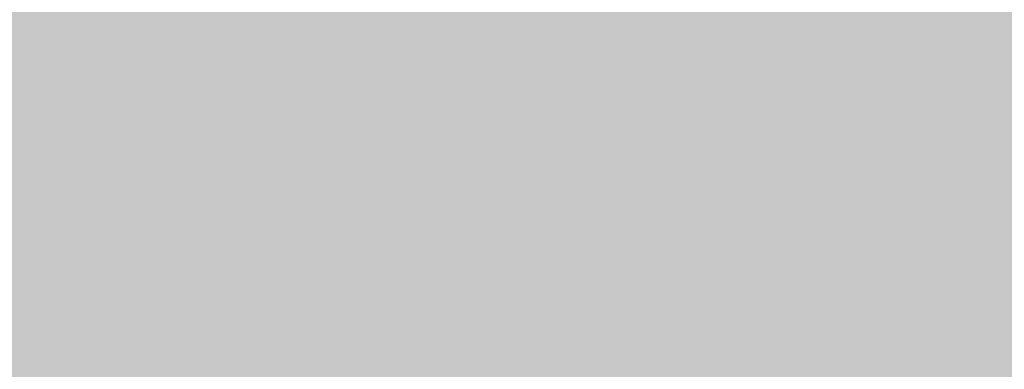
# Model space of a CAD drawing. Units: feet. Extents: x 3168 to 4724, y 827 to 1477.
# Tile 19 of 256: x 3257.497 to 3261.901, y 1096.781 to 1098.344. Entities that reach past the tile are written whole.
import ezdxf

# ---------------------------------------------------------------- set-up
doc = ezdxf.new("R2010")
doc.units = ezdxf.units.FT
doc.layers.add('A-ELEV-PATT', color=8, linetype='Continuous', lineweight=13)

msp = doc.modelspace()

# ---------------------------------------------------------------- hatches: boundary and pattern name
at = {"layer": 'A-ELEV-PATT'}
h = msp.add_hatch(color=256, dxfattribs=at)
h.dxf.hatch_style = 1
edge = h.paths.add_edge_path()
edge.add_ellipse((3552.9058, 979.2201), major_axis=(36.7449, 0), ratio=0.4848485, start_angle=0, end_angle=360)
edge = h.paths.add_edge_path()
edge.add_ellipse((3559.8916, 929.2523), major_axis=(36.7449, 0), ratio=0.4848485, start_angle=0, end_angle=360)
edge = h.paths.add_edge_path()
edge.add_line((3299.3168, 1198.6061), (3479.9167, 1198.6061))
edge.add_line((3479.9167, 1198.6061), (3479.9167, 1209.8686))
edge.add_spline(control_points=[(3479.9167, 1209.8686), (3464.3012, 1209.8686), (3448.6856, 1209.8686), (3410.9491, 1209.8686), (3388.8282, 1209.8686), (3355.6469, 1209.8686), (3344.5864, 1209.8686), (3327.9957, 1209.8686), (3322.4655, 1209.8686), (3314.1702, 1209.8686), (3311.4051, 1209.8686), (3307.2574, 1209.8686), (3305.8748, 1209.8686), (3303.801, 1209.8686), (3303.1097, 1209.8686), (3302.0728, 1209.8686), (3301.7272, 1209.8686), (3301.2087, 1209.8686), (3301.0359, 1209.8686), (3300.7767, 1209.8686), (3300.6903, 1209.8686), (3300.5606, 1209.8686), (3300.5174, 1209.8686), (3300.4526, 1209.8686), (3300.431, 1209.8686), (3300.3986, 1209.8686), (3300.3878, 1209.8686), (3300.3662, 1209.8686), (3300.3457, 1209.8686), (3300.3455, 1209.8686), (3300.3455, 1209.8686), (3300.3433, 1209.8686), (3300.3411, 1209.8686), (3300.3379, 1209.8686), (3300.3368, 1209.8686), (3300.3339, 1209.8686), (3300.3321, 1209.8686), (3300.3255, 1209.8686), (3300.3207, 1209.8686), (3300.3109, 1209.8686), (3300.306, 1209.8686), (3300.2905, 1209.8686), (3300.28, 1209.8686), (3300.2324, 1209.8688), (3300.1953, 1209.869), (3299.9511, 1209.8706), (3299.7448, 1209.8743), (3299.4368, 1209.8833), (3299.3344, 1209.8868), (3299.1811, 1209.8929), (3299.13, 1209.8951), (3298.6522, 1209.9168), (3298.2295, 1209.9457), (3297.6016, 1210.0024), (3297.3934, 1210.0235), (3297.0827, 1210.0583), (3296.9793, 1210.0705), (3296.293, 1210.1549), (3295.7181, 1210.2434), (3294.8687, 1210.3989), (3294.5877, 1210.4545), (3294.1693, 1210.5433), (3294.0304, 1210.5739), (3291.7071, 1211.1012), (3289.6536, 1211.8134), (3285.7763, 1213.564), (3283.9514, 1214.6035), (3280.5122, 1216.9801), (3278.8972, 1218.3176), (3276.3799, 1220.8295), (3275.416, 1221.9177), (3274.0393, 1223.7077), (3273.581, 1224.3495), (3273.1432, 1225.0163)], knot_values=[39.119033, 39.119033, 39.119033, 39.119033, 39.286353, 39.286353, 39.523379, 39.523379, 39.641892, 39.641892, 39.701148, 39.701148, 39.730777, 39.730777, 39.745591, 39.745591, 39.752998, 39.752998, 39.756701, 39.756701, 39.758553, 39.758553, 39.759479, 39.759479, 39.759942, 39.759942, 39.760173, 39.760173, 39.760289, 39.760289, 39.760405, 39.760405, 39.760463, 39.760463, 39.763389, 39.763389, 39.764851, 39.764851, 39.767304, 39.767304, 39.773825, 39.773825, 39.78057, 39.78057, 39.79477, 39.79477, 39.845194, 39.845194, 40.126715, 40.126715, 40.267476, 40.267476, 40.337856, 40.337856, 40.927023, 40.927023, 41.221606, 41.221606, 41.368898, 41.368898, 42.202622, 42.202622, 42.619485, 42.619485, 42.827916, 42.827916, 46.118323, 46.118323, 49.408731, 49.408731, 52.699139, 52.699139, 54.927489, 54.927489, 56.104228, 56.104228, 56.104228, 56.104228], weights=[1, 1, 1, 1, 1, 1, 1, 1, 1, 1, 1, 1, 1, 1, 1, 1, 1, 1, 1, 1, 1, 1, 1, 1, 1, 1, 1, 1, 1, 1, 1, 1, 1, 1, 1, 1, 1, 1, 1, 1, 1, 1, 1, 1, 1, 1, 1, 1, 1, 1, 1, 1, 1, 1, 1, 1, 1, 1, 1, 1, 1, 1, 1, 1, 1, 1, 1, 1, 1, 1, 1, 1, 1, 1], degree=3, periodic=0)
edge.add_line((3273.1432, 1225.0163), (3273.1432, 1099.0163))
edge.add_line((3273.1432, 1099.0163), (3299.3168, 1099.0163))
edge.add_line((3299.3168, 1099.0163), (3299.3168, 1198.6061))
edge = h.paths.add_edge_path()
edge.add_line((3304.7584, 1324.1581), (3479.9167, 1324.1581))
edge.add_line((3479.9167, 1324.1581), (3479.9167, 1335.7146))
edge.add_line((3479.9167, 1335.7146), (3269.1616, 1335.7146))
edge.add_spline(control_points=[(3269.1616, 1335.7146), (3264.0242, 1335.7146), (3258.3641, 1328.9582), (3259.2643, 1323.9003)], knot_values=[0, 0, 0, 0, 15.412191, 15.412191, 15.412191, 15.412191], degree=3, periodic=0)
edge.add_line((3259.2643, 1323.9003), (3265.5168, 1288.7691))
edge.add_line((3265.5168, 1288.7691), (3275.2651, 1261.5456))
edge.add_line((3275.2651, 1261.5456), (3304.7584, 1261.5456))
edge.add_line((3304.7584, 1261.5456), (3304.7584, 1324.1581))
h = msp.add_hatch(color=256, dxfattribs=at)
h.dxf.hatch_style = 1
h.paths.add_polyline_path([(3384.5252, 1099.0163), (3335.0292, 1099.0163), (3299.3168, 1099.0163), (3273.1432, 1099.0163), (3217.5654, 1099.0163), (3168.0693, 827.1163), (3335.0292, 827.1163)])

doc.saveas('drawing.dxf')
